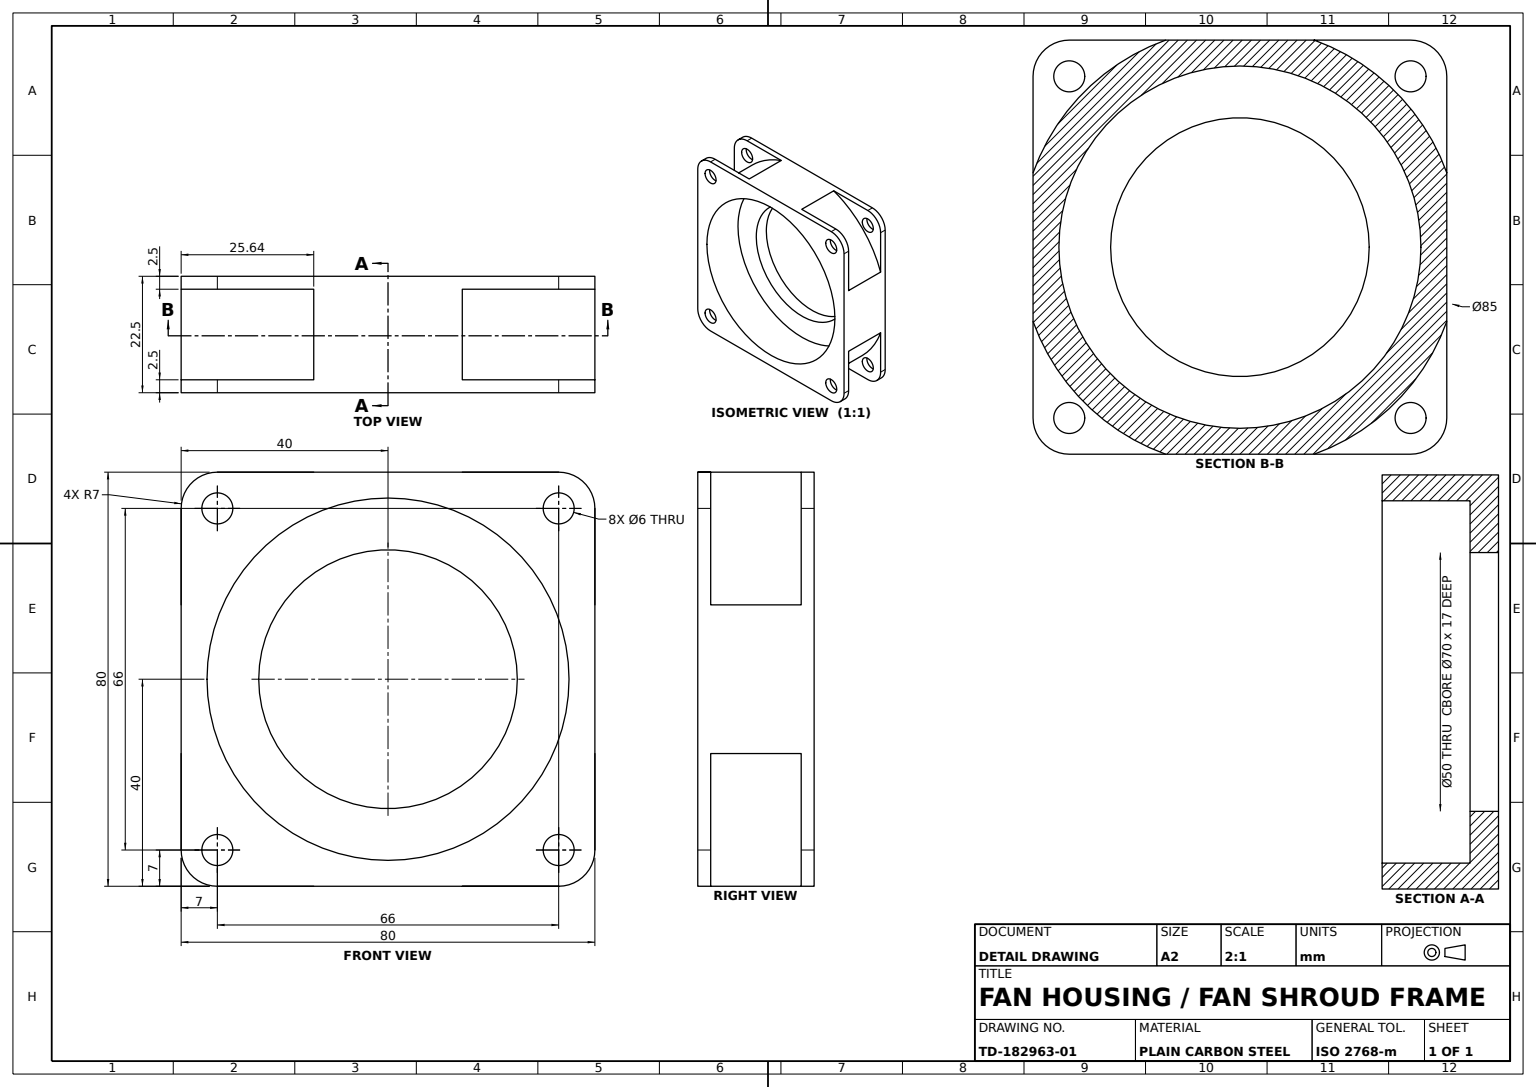
from build123d import *

# Parameters (mm, degrees)
FRONT_FLANGE_80X80_DEPTH = 2.5
HUB_SKETCH_R             = 35
HUB_70_DEPTH             = 20
REAR_START               = -2.5
REAR_FLANGE_80X80_DEPTH  = 2.5
SIDE_WEBS_DEPTH          = 20
LARGE_BORE_SKETCH_R      = 35
LARGE_BORE_70_DEPTH      = 17
THROUGH_BORE_SKETCH_R    = 25
THROUGH_BORE_50_DEPTH    = 8
CORNER_HOLES_SKETCH_R    = 3
CORNER_HOLES_4X_6_DEPTH  = 25


with BuildPart() as part:
    # Front Flange Sketch → Front Flange 80x80 (new body)
    with BuildSketch(Plane.XY):
        with BuildLine():
            Line((0, 0), (33, 0))
            ThreePointArc((33, 0), (37.949747468, 2.050252532), (40, 7))
            Line((40, 7), (40, 73))
            ThreePointArc((40, 73), (37.949747468, 77.949747468), (33, 80))
            Line((33, 80), (-33, 80))
            ThreePointArc((-33, 80), (-37.949747468, 77.949747468), (-40, 73))
            Line((-40, 73), (-40, 7))
            ThreePointArc((-40, 7), (-37.949747468, 2.050252532), (-33, 0))
            Line((-33, 0), (0, 0))
        make_face()
    extrude(amount=FRONT_FLANGE_80X80_DEPTH)

    # Hub Sketch → Hub Ø70 (add)
    with BuildSketch(Plane.XY.offset(2.5)):
        with Locations((0, 40)):
            Circle(HUB_SKETCH_R)
    extrude(amount=HUB_70_DEPTH)

    # Rear Flange Sketch → Rear Flange 80x80 (add)
    with BuildSketch(Plane.XY.offset(22.5).offset(REAR_START)):
        with BuildLine():
            Line((40, 7), (40, 40))
            Line((40, 40), (40, 73))
            ThreePointArc((40, 73), (37.949747468, 77.949747468), (33, 80))
            Line((33, 80), (-33, 80))
            ThreePointArc((-33, 80), (-37.949747468, 77.949747468), (-40, 73))
            Line((-40, 73), (-40, 7))
            ThreePointArc((-40, 7), (-37.949747468, 2.050252532), (-33, 0))
            Line((-33, 0), (33, 0))
            ThreePointArc((33, 0), (37.949747468, 2.050252532), (40, 7))
        make_face()
    extrude(amount=REAR_FLANGE_80X80_DEPTH)

    # Side Web Sketch → Side Webs (add)
    with BuildSketch(Plane.XY.offset(22.5)):
        with BuildLine():
            Line((-14.361406616, 80), (14.361406616, 80))
            ThreePointArc((14.361406616, 80), (30.0520382, 70.0520382), (40, 54.361406616))
            Line((40, 54.361406616), (40, 25.638593384))
            ThreePointArc((40, 25.638593384), (30.0520382, 9.9479618), (14.361406616, 0))
            Line((14.361406616, 0), (-14.361406616, 0))
            ThreePointArc((-14.361406616, 0), (-30.0520382, 9.9479618), (-40, 25.638593384))
            Line((-40, 25.638593384), (-40, 54.361406616))
            ThreePointArc((-40, 54.361406616), (-30.0520382, 70.0520382), (-14.361406616, 80))
        make_face()
    extrude(amount=-SIDE_WEBS_DEPTH)

    # Large Bore Sketch → Large Bore Ø70 (cut)
    with BuildSketch(Plane.XY.offset(22.5)):
        with Locations((0, 40)):
            Circle(LARGE_BORE_SKETCH_R)
    extrude(amount=-LARGE_BORE_70_DEPTH, mode=Mode.SUBTRACT)

    # Through Bore Sketch → Through Bore Ø50 (cut)
    with BuildSketch(Plane.XY.offset(5.5)):
        with Locations((0, 40)):
            Circle(THROUGH_BORE_SKETCH_R)
    extrude(amount=-THROUGH_BORE_50_DEPTH, mode=Mode.SUBTRACT)

    # Corner Holes Sketch → Corner Holes 4xØ6 (cut)
    with BuildSketch(Plane.XY.offset(22.5)):
        with Locations((-33, 73)):
            Circle(CORNER_HOLES_SKETCH_R)
        with Locations((33, 73)):
            Circle(CORNER_HOLES_SKETCH_R)
        with Locations((-33, 7)):
            Circle(CORNER_HOLES_SKETCH_R)
        with Locations((33, 7)):
            Circle(CORNER_HOLES_SKETCH_R)
    extrude(amount=-CORNER_HOLES_4X_6_DEPTH, mode=Mode.SUBTRACT)


solid = part.part
